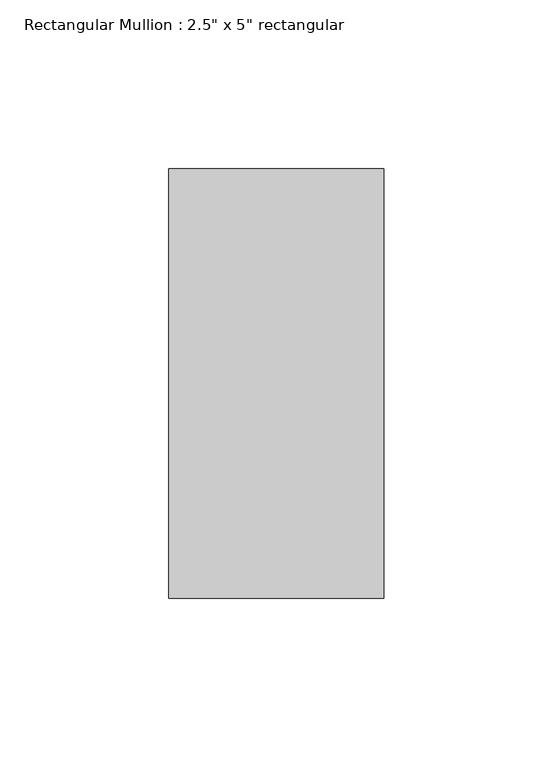
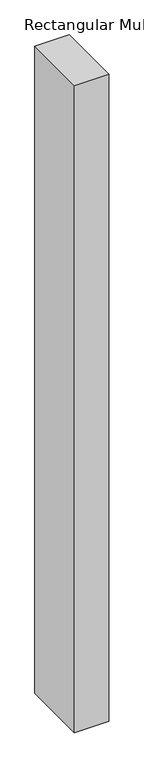
"""IFC4 building model written with IfcOpenShell, lengths in millimetres: member geometry."""

from ifc_helpers import new_model, si_unit, frame, origin, place, context, project, spatial, polyline, outline, extrude, source, transform, mapped, element, save


def member_2b44a902(model_context):
    return source(origin(), model_context, "Body", "SweptSolid", [
        extrude(outline(polyline([(31.75, 63.5), (31.75, -63.5), (-31.75, -63.5), (-31.75, 63.5), (31.75, 63.5)])), frame((0.0, 0.0, -1270.0), z_axis=(0.0, 0.0, 1.0), x_axis=(1.0, 0.0, 0.0)), (0.0, 0.0, 1.0), 1270.0),
    ])


if __name__ == "__main__":
    model = new_model("IFC4")
    model_context = context("Model", 3, world=origin())
    ifc_project = project(units=[si_unit("LENGTHUNIT", "METRE", prefix="MILLI")], contexts=[model_context])
    site = spatial("IfcSite", under=ifc_project)
    building = spatial("IfcBuilding", under=site)
    placement = place(None, origin())
    member_shape = member_2b44a902(model_context)
    element("IfcMember", 1, ObjectType="Rectangular Mullion : 2.5\" x 5\" rectangular", at=placement, inside=building, context=model_context, shape_type="MappedRepresentation", body=[
        mapped(member_shape, transform((0.0, 0.0, 0.0), x_axis=(1.0, 0.0, 0.0), y_axis=(0.0, 1.0, 0.0), z_axis=(0.0, 0.0, 1.0))),
    ])
    save(model, "model.ifc")

# Revit data of these elements
# Type "Rectangular Mullion : 2.5\" x 5\" rectangular"
#   built-in parameter 1007304 = 0.416667 (stored number, unit not read)
#   built-in parameter 1007301 = 0.104167 (stored number, unit not read)
#   built-in parameter 1007300 = 0.104167 (stored number, unit not read)
